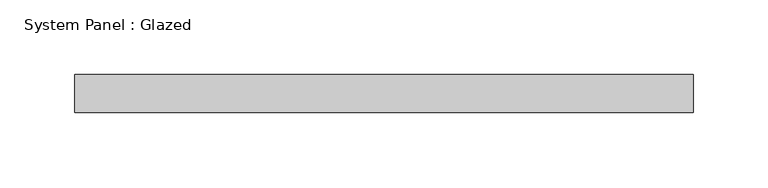
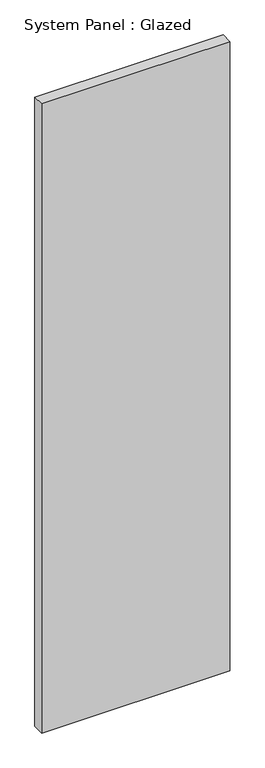
"""IFC4 building model written with IfcOpenShell, lengths in millimetres: plate geometry, System Panel : Glazed."""

from ifc_helpers import new_model, si_unit, origin, origin_with_axes, place, context, project, spatial, polyline, outline, extrude, source, transform, mapped, element, save


def system_panel_glazed_5eb5e9ea(model_context):
    return source(origin(), model_context, "Body", "SweptSolid", [
        extrude(outline(polyline([(206.375, 19.05), (-206.375, 19.05), (-206.375, 44.45), (206.375, 44.45), (206.375, 19.05)])), origin_with_axes(), (0.0, 0.0, 1.0), 1459.2856263),
    ])


if __name__ == "__main__":
    model = new_model("IFC4")
    model_context = context("Model", 3, world=origin())
    ifc_project = project(units=[si_unit("LENGTHUNIT", "METRE", prefix="MILLI")], contexts=[model_context])
    site = spatial("IfcSite", under=ifc_project)
    building = spatial("IfcBuilding", under=site)
    placement = place(None, origin())
    system_panel_glazed_shape = system_panel_glazed_5eb5e9ea(model_context)
    element("IfcPlate", 1, ObjectType="System Panel : Glazed", at=placement, inside=building, context=model_context, shape_type="MappedRepresentation", body=[
        mapped(system_panel_glazed_shape, transform((0.0, 0.0, 0.0), x_axis=(1.0, 0.0, 0.0), y_axis=(0.0, 1.0, 0.0), z_axis=(0.0, 0.0, 1.0))),
    ])
    save(model, "model.ifc")

# Revit data of these elements
# Type "System Panel : Glazed"
#   Construction Type Id = "GSP4R"
#   Analytic Construction = "1/8 in Pilkington single glazing"
#   Visual Light Transmittance = 0.9
#   Solar Heat Gain Coefficient = 0.86
#   Heat Transfer Coefficient (U) = 1.18115 BTU/(h·ft²·°F)
#   Define Thermal Properties by = 1
# Element 1 (IfcPlate, "System Panel : Glazed")
#   Materials on its faces: "Glass"
# Materials
#   "Glass": class "Glass", colour RGB 0 128 192, transparency 0.75, Description = "Soda Lime Glass", Cost = 0
